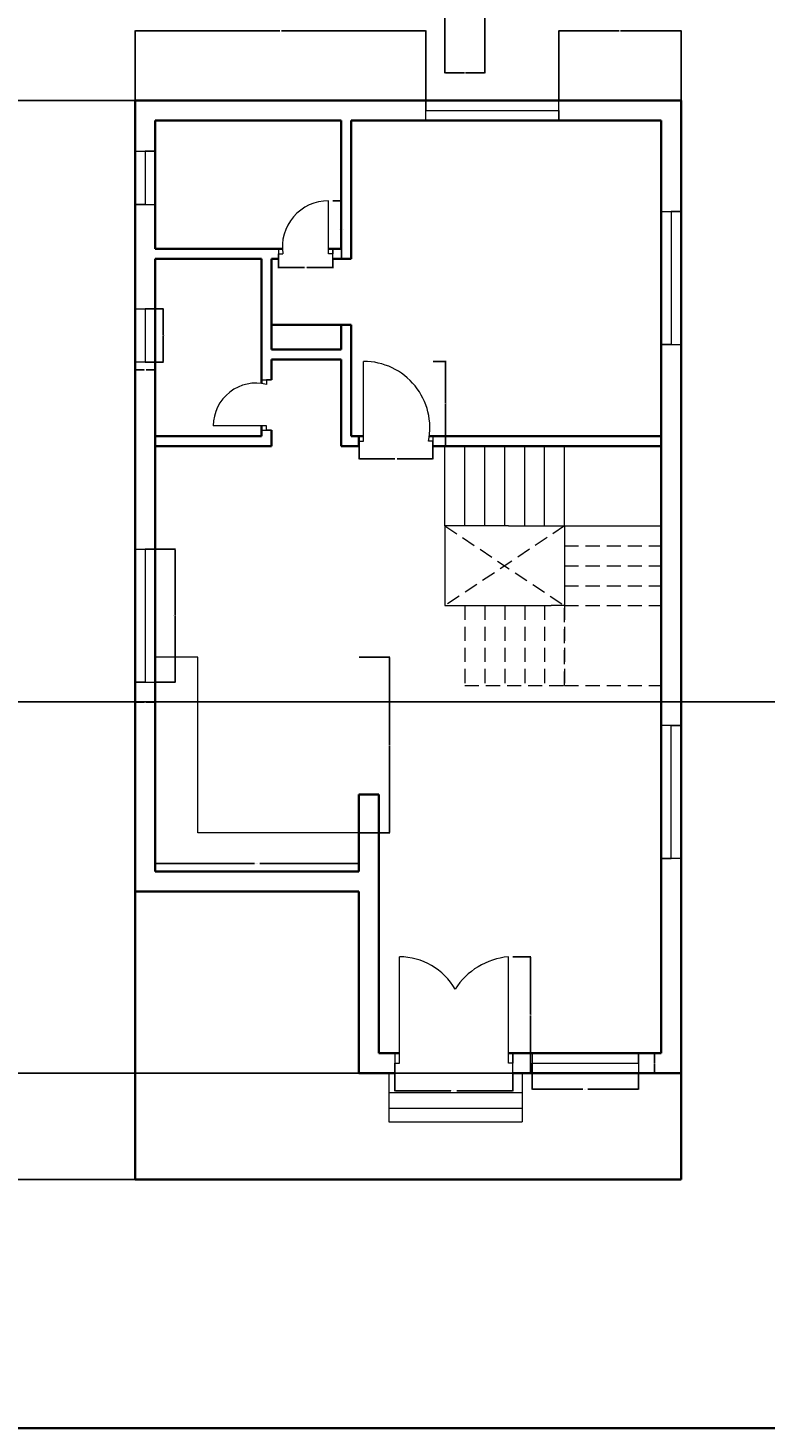
# Model space of a CAD drawing. Units: inches. Extents: x 1911 to 3278, y 2022 to 3108.
# Tile 11 of 13: x 2585 to 2918, y 2022 to 2654. Entities that reach past the tile are written whole.
import ezdxf

# ---------------------------------------------------------------- set-up
doc = ezdxf.new("R2010")
doc.units = ezdxf.units.IN
doc.linetypes.add('DASHED2', pattern=[9.525, 6.35, -3.175])
for name, color, linetype, lineweight in [('A-ANNO-DIMS', 2, 'Continuous', 18), ('A-ANNO-SYMB', 7, 'Continuous', 25), ('A-ANNO-TTLB', 7, 'Continuous', 35), ('A-DOOR', 4, 'Continuous', 18), ('A-FLOR-CASE', 9, 'Continuous', 18), ('A-FLOR-STRS', 7, 'Continuous', 18), ('A-FLOR-STRS-OVHD', 253, 'DASHED2', 13), ('A-GLAZ', 4, 'Continuous', 18), ('A-WALL', 7, 'Continuous', 35)]:
    doc.layers.add(name, color=color, linetype=linetype, lineweight=lineweight)
doc.styles.get("Standard").update_dxf_attribs({"font": 'arial.ttf'})
doc.dimstyles.get("Standard").update_dxf_attribs({"dimtxt": 0.18, "dimasz": 0.18, "dimexe": 0.18, "dimexo": 0.0625, "dimgap": 0.09, "dimtad": 0, "dimtih": 1, "dimtoh": 1, "dimdec": 4, "dimzin": 0, "dimdsep": 46, "dimtxsty": 'Standard', "dimcen": 0.09, "dimadec": 0, "dimazin": 0, "dimtfac": 1, "dimtdec": 4, "dimtofl": 0, "dimtmove": 0, "dimatfit": 3, "dimfxl": 1, "dimtolj": 1, "dimtzin": 0, "dimarcsym": 0})

# ---------------------------------------------------------------- blocks, each defined once
blk = doc.blocks.new('WIN-60')
for p, q in [((0, 60), (9, 60)), ((9, 60), (4.5, 60)), ((4.5, 60), (4.5, 0)), ((4.5, 0), (0, 0)), ((0, 0), (9, 0))]:
    blk.add_line(p, q)
blk = doc.blocks.new('WIN-24')
for p, q in [((0, 24), (9, 24)), ((9, 24), (4.5, 24)), ((4.5, 24), (4.5, 0)), ((4.5, 0), (0, 0)), ((0, 0), (9, 0))]:
    blk.add_line(p, q)
blk = doc.blocks.new('WIN-24-ALT-JAMB')
for p, q in [((0, 24), (9, 24)), ((9, 24), (4.5, 24)), ((4.5, 24), (4.5, 0)), ((9, 0), (0, 0)), ((4.5, 0), (9, 0))]:
    blk.add_line(p, q)
blk = doc.blocks.new('WIN-48')
for p, q in [((0, 9), (0, 0)), ((48, 4.5), (48, 9)), ((48, 9), (48, 0)), ((0, 0), (0, 4.5)), ((0, 4.5), (36, 4.5)), ((36, 4.5), (48, 4.5))]:
    blk.add_line(p, q)
blk = doc.blocks.new('DOOR-BATH-GF')
for p, q in [((22.54, 2.25), (22.54, 26.25)), ((0, 4.5), (0, 0)), ((0, 0), (0, 2.25)), ((0, 2.25), (2, 2.25)), ((24.54, 2.25), (22.54, 2.25)), ((24.54, 0), (24.54, 4.5)), ((24.54, 4.5), (24.54, 2.25))]:
    blk.add_line(p, q)
blk.add_arc((22.54, 5.46), 20.79, 90, 188.87385)
blk = doc.blocks.new('DOOR-WC-GF')
for p, q in [((21.75, 22.69), (26.25, 22.69)), ((26.25, 22.69), (24, 22.69)), ((24, 22.69), (24, 20.69)), ((24, 2), (0, 2)), ((24, 0), (24, 2)), ((21.75, 0), (26.25, 0)), ((26.25, 0), (24, 0))]:
    blk.add_line(p, q)
blk.add_arc((19.28, 2), 19.28, 75.82669, 180)
blk = doc.blocks.new('DOOR-BED-GF')
for p, q in [((2, 2.25), (2, 38.25)), ((0, 4.5), (0, 0)), ((0, 0), (0, 2.25)), ((0, 2.25), (0, 2.25)), ((0, 2.25), (2, 2.25)), ((33.28, 2.25), (31.28, 2.25)), ((33.28, 4.5), (33.28, 0)), ((33.28, 0), (33.28, 2.25))]:
    blk.add_line(p, q)
blk.add_arc((2, 8.34), 29.91, 348.25045, 90)
blk = doc.blocks.new('DOOR-ENTRY-PAIR')
for p, q in [((2, 40.5), (2, 52.5)), ((51.21, 4.5), (51.21, 52.5)), ((2, 4.5), (2, 40.5)), ((0, 9), (0, 0)), ((53.21, 0), (53.21, 9)), ((53.21, 9), (53.21, 4.5)), ((0, 0), (0, 4.5)), ((0, 4.5), (2, 4.5)), ((53.21, 4.5), (51.21, 4.5))]:
    blk.add_line(p, q)
for centre, radius, start, end in [((2, 23.47), 29.03, 29.81913, 90), ((54.01, 20.81), 31.81, 95.05335, 147.49255)]:
    blk.add_arc(centre, radius, start, end)
blk = doc.blocks.new('STEPS-ENTRY')
for p, q in [((0, 21.91), (0, 0)), ((60.1, 21.91), (60.1, 0)), ((0, 13.22), (60.1, 13.22)), ((60.1, 13.22), (60.1, 6)), ((60.1, 6), (0, 6)), ((0, 6), (0, 0)), ((0, 0), (60.1, 0))]:
    blk.add_line(p, q)
blk = doc.blocks.new('COUNTER-KITCHEN-L')
for p, q in [((19.27, 79.32), (0, 79.32)), ((19.27, 0), (19.27, 79.32)), ((92, 0), (19.27, 0))]:
    blk.add_line(p, q)
blk = doc.blocks.new('STAIR-PLAN-GF')
for p, q in [((0, 36), (0, 72)), ((9, 36), (9, 72)), ((18, 36), (18, 72)), ((27, 36), (27, 72)), ((36, 36), (36, 72)), ((45, 36), (45, 72)), ((54, 36), (54, 72)), ((28.63, 36), (0, 36)), ((0, 36), (0, 0)), ((28.63, 36), (97.65, 36)), ((54, 36), (54, 0)), ((54, 36), (54, 27)), ((0, 0), (48, 0)), ((54, 0), (48, 0))]:
    blk.add_line(p, q)
blk = doc.blocks.new('STAIR-BEYOND-GF')
for p, q in [((54, 72), (0, 36)), ((0, 72), (54, 36)), ((54, 72), (54, 63)), ((54, 63), (97.65, 63)), ((54, 54), (97.65, 54)), ((54, 45), (97.65, 45)), ((9, 36), (9, 0)), ((18, 36), (18, 0)), ((27, 36), (27, 0)), ((36, 36), (36, 0)), ((45, 36), (45, 0)), ((54, 36), (97.65, 36)), ((54, 0), (54, 36)), ((54, 36), (54, 0)), ((9, 0), (54, 0)), ((54, 0), (97.65, 0))]:
    blk.add_line(p, q)
blk = doc.blocks.new('*D24')
at = {"layer": 'A-ANNO-DIMS', "color": 0, "lineweight": -2, "transparency": 16777216}
for p, q in [((2642.42, 2418.3), (2651.53, 2418.3)), ((2651.35, 2418.12), (2651.35, 2388.48)), ((2651.35, 2358.48), (2651.35, 2388.12)), ((2642.42, 2358.3), (2651.53, 2358.3))]:
    blk.add_line(p, q, dxfattribs=at)
at = {"layer": 'A-ANNO-DIMS', "color": 0, "transparency": 16777216}
for points in [[(2651.32, 2418.12), (2651.38, 2418.12), (2651.35, 2418.3)], [(2651.32, 2358.48), (2651.38, 2358.48), (2651.35, 2358.3)]]:
    blk.add_solid(points, dxfattribs=at)
at = {"layer": 'Defpoints', "color": 0, "transparency": 16777216}
for p in [(2642.35, 2418.3), (2651.35, 2418.3), (2642.35, 2358.3)]:
    blk.add_point(p, dxfattribs=at)
at = {"layer": 'A-ANNO-DIMS', "color": 0, "transparency": 16777216, "insert": (2651.35, 2388.3), "char_height": 0.18, "attachment_point": 5}
blk.add_mtext('\\A1;WINDOW 60 TYP.', dxfattribs=at)
blk = doc.blocks.new('*D25')
at = {"layer": 'A-ANNO-DIMS', "color": 0, "lineweight": -2, "transparency": 16777216}
for p, q in [((2633.35, 2358.24), (2633.35, 2349.12)), ((2642.35, 2358.24), (2642.35, 2349.12)), ((2633.53, 2349.3), (2637.4, 2349.3)), ((2642.17, 2349.3), (2638.31, 2349.3))]:
    blk.add_line(p, q, dxfattribs=at)
at = {"layer": 'A-ANNO-DIMS', "color": 0, "transparency": 16777216}
for points in [[(2633.53, 2349.33), (2633.53, 2349.27), (2633.35, 2349.3)], [(2642.17, 2349.33), (2642.17, 2349.27), (2642.35, 2349.3)]]:
    blk.add_solid(points, dxfattribs=at)
at = {"layer": 'Defpoints', "color": 0, "transparency": 16777216}
for p in [(2633.35, 2358.3), (2642.35, 2358.3), (2642.35, 2349.3)]:
    blk.add_point(p, dxfattribs=at)
at = {"layer": 'A-ANNO-DIMS', "color": 0, "transparency": 16777216, "insert": (2637.85, 2349.3), "char_height": 0.18, "attachment_point": 5}
blk.add_mtext('\\A1;9 TYP.', dxfattribs=at)
blk = doc.blocks.new('*D28')
at = {"layer": 'A-ANNO-DIMS', "color": 0, "lineweight": -2, "transparency": 16777216}
for p, q in [((2642.42, 2526.84), (2646.13, 2526.84)), ((2645.95, 2526.66), (2645.95, 2515.02)), ((2645.95, 2503.02), (2645.95, 2514.66)), ((2642.42, 2502.84), (2646.13, 2502.84))]:
    blk.add_line(p, q, dxfattribs=at)
at = {"layer": 'A-ANNO-DIMS', "color": 0, "transparency": 16777216}
for points in [[(2645.92, 2526.66), (2645.98, 2526.66), (2645.95, 2526.84)], [(2645.92, 2503.02), (2645.98, 2503.02), (2645.95, 2502.84)]]:
    blk.add_solid(points, dxfattribs=at)
at = {"layer": 'Defpoints', "color": 0, "transparency": 16777216}
for p in [(2642.35, 2526.84), (2645.95, 2526.84), (2642.35, 2502.84)]:
    blk.add_point(p, dxfattribs=at)
at = {"layer": 'A-ANNO-DIMS', "color": 0, "transparency": 16777216, "insert": (2645.95, 2514.84), "char_height": 0.18, "attachment_point": 5}
blk.add_mtext('\\A1;ALT. JAMB 24 TYP.', dxfattribs=at)
blk = doc.blocks.new('*D29')
at = {"layer": 'A-ANNO-DIMS', "color": 0, "lineweight": -2, "transparency": 16777216}
for p, q in [((2633.35, 2502.78), (2633.35, 2499.06)), ((2642.35, 2502.78), (2642.35, 2499.06)), ((2633.53, 2499.24), (2637.4, 2499.24)), ((2642.17, 2499.24), (2638.31, 2499.24))]:
    blk.add_line(p, q, dxfattribs=at)
at = {"layer": 'A-ANNO-DIMS', "color": 0, "transparency": 16777216}
for points in [[(2633.53, 2499.27), (2633.53, 2499.21), (2633.35, 2499.24)], [(2642.17, 2499.27), (2642.17, 2499.21), (2642.35, 2499.24)]]:
    blk.add_solid(points, dxfattribs=at)
at = {"layer": 'Defpoints', "color": 0, "transparency": 16777216}
for p in [(2633.35, 2502.84), (2642.35, 2502.84), (2642.35, 2499.24)]:
    blk.add_point(p, dxfattribs=at)
at = {"layer": 'A-ANNO-DIMS', "color": 0, "transparency": 16777216, "insert": (2637.85, 2499.24), "char_height": 0.18, "attachment_point": 5}
blk.add_mtext('\\A1;9 TYP.', dxfattribs=at)
blk = doc.blocks.new('*D30')
at = {"layer": 'A-ANNO-DIMS', "color": 0, "lineweight": -2, "transparency": 16777216}
for p, q in [((2812.56, 2181.81), (2812.56, 2174.49)), ((2860.56, 2181.81), (2860.56, 2174.49)), ((2812.74, 2174.67), (2835.44, 2174.67)), ((2860.38, 2174.67), (2837.68, 2174.67))]:
    blk.add_line(p, q, dxfattribs=at)
at = {"layer": 'A-ANNO-DIMS', "color": 0, "transparency": 16777216}
for points in [[(2812.74, 2174.7), (2812.74, 2174.64), (2812.56, 2174.67)], [(2860.38, 2174.7), (2860.38, 2174.64), (2860.56, 2174.67)]]:
    blk.add_solid(points, dxfattribs=at)
at = {"layer": 'Defpoints', "color": 0, "transparency": 16777216}
for p in [(2812.56, 2181.87), (2860.56, 2181.87), (2860.56, 2174.67)]:
    blk.add_point(p, dxfattribs=at)
at = {"layer": 'A-ANNO-DIMS', "color": 0, "transparency": 16777216, "insert": (2836.56, 2174.67), "char_height": 0.18, "attachment_point": 5}
blk.add_mtext('\\A1;WINDOW 48 TYP.', dxfattribs=at)
blk = doc.blocks.new('*D31')
at = {"layer": 'A-ANNO-DIMS', "color": 0, "lineweight": -2, "transparency": 16777216}
for p, q in [((2860.62, 2190.87), (2867.94, 2190.87)), ((2867.76, 2190.69), (2867.76, 2186.56)), ((2860.62, 2181.87), (2867.94, 2181.87)), ((2867.76, 2182.05), (2867.76, 2186.19))]:
    blk.add_line(p, q, dxfattribs=at)
at = {"layer": 'A-ANNO-DIMS', "color": 0, "transparency": 16777216}
for points in [[(2867.73, 2190.69), (2867.79, 2190.69), (2867.76, 2190.87)], [(2867.73, 2182.05), (2867.79, 2182.05), (2867.76, 2181.87)]]:
    blk.add_solid(points, dxfattribs=at)
at = {"layer": 'Defpoints', "color": 0, "transparency": 16777216}
for p in [(2860.56, 2190.87), (2867.76, 2190.87), (2860.56, 2181.87)]:
    blk.add_point(p, dxfattribs=at)
at = {"layer": 'A-ANNO-DIMS', "color": 0, "transparency": 16777216, "insert": (2867.76, 2186.37), "char_height": 0.18, "attachment_point": 5}
blk.add_mtext('\\A1;9 TYP.', dxfattribs=at)
blk = doc.blocks.new('*D38')
at = {"layer": 'A-ANNO-DIMS', "color": 0, "lineweight": -2, "transparency": 16777216}
for p, q in [((2722.63, 2575.62), (2726.69, 2575.62)), ((2726.51, 2575.44), (2726.51, 2562.68)), ((2726.51, 2549.55), (2726.51, 2562.32)), ((2722.63, 2549.37), (2726.69, 2549.37))]:
    blk.add_line(p, q, dxfattribs=at)
at = {"layer": 'A-ANNO-DIMS', "color": 0, "transparency": 16777216}
for points in [[(2726.48, 2575.44), (2726.54, 2575.44), (2726.51, 2575.62)], [(2726.48, 2549.55), (2726.54, 2549.55), (2726.51, 2549.37)]]:
    blk.add_solid(points, dxfattribs=at)
at = {"layer": 'Defpoints', "color": 0, "transparency": 16777216}
for p in [(2722.57, 2575.62), (2726.51, 2575.62), (2722.57, 2549.37)]:
    blk.add_point(p, dxfattribs=at)
at = {"layer": 'A-ANNO-DIMS', "color": 0, "transparency": 16777216, "insert": (2726.51, 2562.5), "char_height": 0.18, "attachment_point": 5}
blk.add_mtext('\\A1;BATH DOOR 26 TYP.', dxfattribs=at)
blk = doc.blocks.new('*D39')
at = {"layer": 'A-ANNO-DIMS', "color": 0, "lineweight": -2, "transparency": 16777216}
for p, q in [((2698.03, 2549.31), (2698.03, 2545.26)), ((2722.57, 2549.31), (2722.57, 2545.26)), ((2698.21, 2545.44), (2709.77, 2545.44)), ((2722.39, 2545.44), (2710.83, 2545.44))]:
    blk.add_line(p, q, dxfattribs=at)
at = {"layer": 'A-ANNO-DIMS', "color": 0, "transparency": 16777216}
for points in [[(2698.21, 2545.47), (2698.21, 2545.41), (2698.03, 2545.44)], [(2722.39, 2545.47), (2722.39, 2545.41), (2722.57, 2545.44)]]:
    blk.add_solid(points, dxfattribs=at)
at = {"layer": 'Defpoints', "color": 0, "transparency": 16777216}
for p in [(2698.03, 2549.37), (2722.57, 2549.37), (2722.57, 2545.44)]:
    blk.add_point(p, dxfattribs=at)
at = {"layer": 'A-ANNO-DIMS', "color": 0, "transparency": 16777216, "insert": (2710.3, 2545.44), "char_height": 0.18, "attachment_point": 5}
blk.add_mtext('\\A1;25 TYP.', dxfattribs=at)
blk = doc.blocks.new('*D42')
at = {"layer": 'A-ANNO-DIMS', "color": 0, "lineweight": -2, "transparency": 16777216}
for p, q in [((2767.82, 2503.12), (2773.67, 2503.12)), ((2773.49, 2502.94), (2773.49, 2484.18)), ((2773.49, 2465.05), (2773.49, 2483.82)), ((2767.82, 2464.87), (2773.67, 2464.87))]:
    blk.add_line(p, q, dxfattribs=at)
at = {"layer": 'A-ANNO-DIMS', "color": 0, "transparency": 16777216}
for points in [[(2773.46, 2502.94), (2773.52, 2502.94), (2773.49, 2503.12)], [(2773.46, 2465.05), (2773.52, 2465.05), (2773.49, 2464.87)]]:
    blk.add_solid(points, dxfattribs=at)
at = {"layer": 'Defpoints', "color": 0, "transparency": 16777216}
for p in [(2767.76, 2503.12), (2773.49, 2503.12), (2767.76, 2464.87)]:
    blk.add_point(p, dxfattribs=at)
at = {"layer": 'A-ANNO-DIMS', "color": 0, "transparency": 16777216, "insert": (2773.49, 2484), "char_height": 0.18, "attachment_point": 5}
blk.add_mtext('\\A1;BEDROOM DOOR 38 TYP.', dxfattribs=at)
blk = doc.blocks.new('*D43')
at = {"layer": 'A-ANNO-DIMS', "color": 0, "lineweight": -2, "transparency": 16777216}
for p, q in [((2734.47, 2464.81), (2734.47, 2458.96)), ((2767.76, 2464.81), (2767.76, 2458.96)), ((2734.65, 2459.14), (2750.59, 2459.14)), ((2767.58, 2459.14), (2751.64, 2459.14))]:
    blk.add_line(p, q, dxfattribs=at)
at = {"layer": 'A-ANNO-DIMS', "color": 0, "transparency": 16777216}
for points in [[(2734.65, 2459.17), (2734.65, 2459.11), (2734.47, 2459.14)], [(2767.58, 2459.17), (2767.58, 2459.11), (2767.76, 2459.14)]]:
    blk.add_solid(points, dxfattribs=at)
at = {"layer": 'Defpoints', "color": 0, "transparency": 16777216}
for p in [(2734.47, 2464.87), (2767.76, 2464.87), (2767.76, 2459.14)]:
    blk.add_point(p, dxfattribs=at)
at = {"layer": 'A-ANNO-DIMS', "color": 0, "transparency": 16777216, "insert": (2751.12, 2459.14), "char_height": 0.18, "attachment_point": 5}
blk.add_mtext('\\A1;33 TYP.', dxfattribs=at)
blk = doc.blocks.new('*D44')
at = {"layer": 'A-ANNO-DIMS', "color": 0, "lineweight": -2, "transparency": 16777216}
for p, q in [((2750.62, 2181.81), (2750.62, 2173.71)), ((2803.83, 2181.81), (2803.83, 2173.71)), ((2750.8, 2173.89), (2775.92, 2173.89)), ((2803.65, 2173.89), (2778.54, 2173.89))]:
    blk.add_line(p, q, dxfattribs=at)
at = {"layer": 'A-ANNO-DIMS', "color": 0, "transparency": 16777216}
for points in [[(2750.8, 2173.92), (2750.8, 2173.86), (2750.62, 2173.89)], [(2803.65, 2173.92), (2803.65, 2173.86), (2803.83, 2173.89)]]:
    blk.add_solid(points, dxfattribs=at)
at = {"layer": 'Defpoints', "color": 0, "transparency": 16777216}
for p in [(2750.62, 2181.87), (2803.83, 2181.87), (2803.83, 2173.89)]:
    blk.add_point(p, dxfattribs=at)
at = {"layer": 'A-ANNO-DIMS', "color": 0, "transparency": 16777216, "insert": (2777.23, 2173.89), "char_height": 0.18, "attachment_point": 5}
blk.add_mtext('\\A1;ENTRY PAIR 53 TYP.', dxfattribs=at)
blk = doc.blocks.new('*D45')
at = {"layer": 'A-ANNO-DIMS', "color": 0, "lineweight": -2, "transparency": 16777216}
for p, q in [((2803.9, 2234.37), (2812, 2234.37)), ((2811.82, 2234.19), (2811.82, 2208.31)), ((2811.82, 2182.05), (2811.82, 2207.94)), ((2803.9, 2181.87), (2812, 2181.87))]:
    blk.add_line(p, q, dxfattribs=at)
at = {"layer": 'A-ANNO-DIMS', "color": 0, "transparency": 16777216}
for points in [[(2811.79, 2234.19), (2811.85, 2234.19), (2811.82, 2234.37)], [(2811.79, 2182.05), (2811.85, 2182.05), (2811.82, 2181.87)]]:
    blk.add_solid(points, dxfattribs=at)
at = {"layer": 'Defpoints', "color": 0, "transparency": 16777216}
for p in [(2803.83, 2234.37), (2811.82, 2234.37), (2803.83, 2181.87)]:
    blk.add_point(p, dxfattribs=at)
at = {"layer": 'A-ANNO-DIMS', "color": 0, "transparency": 16777216, "insert": (2811.82, 2208.12), "char_height": 0.18, "attachment_point": 5}
blk.add_mtext('\\A1;53 TYP.', dxfattribs=at)
blk = doc.blocks.new('*D58')
at = {"layer": 'A-ANNO-DIMS', "color": 0, "lineweight": -2, "transparency": 16777216}
for p, q in [((2642.35, 2290.21), (2642.35, 2276.29)), ((2734.35, 2290.21), (2734.35, 2276.29)), ((2642.53, 2276.47), (2687.17, 2276.47)), ((2734.17, 2276.47), (2689.54, 2276.47))]:
    blk.add_line(p, q, dxfattribs=at)
at = {"layer": 'A-ANNO-DIMS', "color": 0, "transparency": 16777216}
for points in [[(2642.53, 2276.5), (2642.53, 2276.44), (2642.35, 2276.47)], [(2734.17, 2276.5), (2734.17, 2276.44), (2734.35, 2276.47)]]:
    blk.add_solid(points, dxfattribs=at)
at = {"layer": 'Defpoints', "color": 0, "transparency": 16777216}
for p in [(2642.35, 2290.27), (2734.35, 2290.27), (2734.35, 2276.47)]:
    blk.add_point(p, dxfattribs=at)
at = {"layer": 'A-ANNO-DIMS', "color": 0, "transparency": 16777216, "insert": (2688.35, 2276.47), "char_height": 0.18, "attachment_point": 5}
blk.add_mtext('\\A1;COUNTER 92 TYP.', dxfattribs=at)
blk = doc.blocks.new('*D59')
at = {"layer": 'A-ANNO-DIMS', "color": 0, "lineweight": -2, "transparency": 16777216}
for p, q in [((2734.42, 2369.59), (2748.33, 2369.59)), ((2748.15, 2369.41), (2748.15, 2330.11)), ((2748.15, 2290.45), (2748.15, 2329.75)), ((2734.42, 2290.27), (2748.33, 2290.27))]:
    blk.add_line(p, q, dxfattribs=at)
at = {"layer": 'A-ANNO-DIMS', "color": 0, "transparency": 16777216}
for points in [[(2748.12, 2369.41), (2748.18, 2369.41), (2748.15, 2369.59)], [(2748.12, 2290.45), (2748.18, 2290.45), (2748.15, 2290.27)]]:
    blk.add_solid(points, dxfattribs=at)
at = {"layer": 'Defpoints', "color": 0, "transparency": 16777216}
for p in [(2734.35, 2369.59), (2748.15, 2369.59), (2734.35, 2290.27)]:
    blk.add_point(p, dxfattribs=at)
at = {"layer": 'A-ANNO-DIMS', "color": 0, "transparency": 16777216, "insert": (2748.15, 2329.93), "char_height": 0.18, "attachment_point": 5}
blk.add_mtext('\\A1;79 TYP.', dxfattribs=at)
blk = doc.blocks.new('*D81')
at = {"layer": 'A-ANNO-DIMS', "color": 0, "lineweight": -2, "transparency": 16777216}
for p, q in [((2633.35, 2620.94), (2633.35, 2652.45)), ((2633.53, 2652.27), (2698.57, 2652.27)), ((2764.37, 2652.27), (2699.34, 2652.27)), ((2764.55, 2620.94), (2764.55, 2652.45))]:
    blk.add_line(p, q, dxfattribs=at)
at = {"layer": 'A-ANNO-DIMS', "color": 0, "transparency": 16777216}
for points in [[(2633.53, 2652.3), (2633.53, 2652.24), (2633.35, 2652.27)], [(2764.37, 2652.3), (2764.37, 2652.24), (2764.55, 2652.27)]]:
    blk.add_solid(points, dxfattribs=at)
at = {"layer": 'Defpoints', "color": 0, "transparency": 16777216}
for p in [(2764.55, 2652.27), (2633.35, 2620.87), (2764.55, 2620.87)]:
    blk.add_point(p, dxfattribs=at)
at = {"layer": 'A-ANNO-DIMS', "color": 0, "transparency": 16777216, "insert": (2698.95, 2652.27), "char_height": 0.18, "attachment_point": 5}
blk.add_mtext('\\A1;131.2', dxfattribs=at)
blk = doc.blocks.new('*D82')
at = {"layer": 'A-ANNO-DIMS', "color": 0, "lineweight": -2, "transparency": 16777216}
for p, q in [((2824.55, 2620.94), (2824.55, 2652.45)), ((2824.73, 2652.27), (2851.88, 2652.27)), ((2879.67, 2652.27), (2852.53, 2652.27)), ((2879.85, 2620.94), (2879.85, 2652.45))]:
    blk.add_line(p, q, dxfattribs=at)
at = {"layer": 'A-ANNO-DIMS', "color": 0, "transparency": 16777216}
for points in [[(2824.73, 2652.3), (2824.73, 2652.24), (2824.55, 2652.27)], [(2879.67, 2652.3), (2879.67, 2652.24), (2879.85, 2652.27)]]:
    blk.add_solid(points, dxfattribs=at)
at = {"layer": 'Defpoints', "color": 0, "transparency": 16777216}
for p in [(2879.85, 2652.27), (2824.55, 2620.87), (2879.85, 2620.87)]:
    blk.add_point(p, dxfattribs=at)
at = {"layer": 'A-ANNO-DIMS', "color": 0, "transparency": 16777216, "insert": (2852.2, 2652.27), "char_height": 0.18, "attachment_point": 5}
blk.add_mtext('\\A1;55.3', dxfattribs=at)
blk = doc.blocks.new('*D83')
at = {"layer": 'A-ANNO-DIMS', "color": 0, "lineweight": -2, "transparency": 16777216}
for p, q in [((2633.29, 2620.87), (2561.76, 2620.87)), ((2561.94, 2620.69), (2561.94, 2485.38)), ((2561.94, 2349.71), (2561.94, 2485.02)), ((2593.28, 2349.53), (2561.76, 2349.53))]:
    blk.add_line(p, q, dxfattribs=at)
at = {"layer": 'A-ANNO-DIMS', "color": 0, "transparency": 16777216}
for points in [[(2561.91, 2620.69), (2561.97, 2620.69), (2561.94, 2620.87)], [(2561.91, 2349.71), (2561.97, 2349.71), (2561.94, 2349.53)]]:
    blk.add_solid(points, dxfattribs=at)
at = {"layer": 'Defpoints', "color": 0, "transparency": 16777216}
for p in [(2561.94, 2620.87), (2633.35, 2620.87), (2593.34, 2349.53)]:
    blk.add_point(p, dxfattribs=at)
at = {"layer": 'A-ANNO-DIMS', "color": 0, "transparency": 16777216, "insert": (2561.94, 2485.2), "char_height": 0.18, "attachment_point": 5}
blk.add_mtext('\\A1;271.35', dxfattribs=at)
blk = doc.blocks.new('*D87')
at = {"layer": 'A-ANNO-DIMS', "color": 0, "lineweight": -2, "transparency": 16777216}
for p, q in [((2593.28, 2349.53), (2561.76, 2349.53)), ((2561.94, 2349.35), (2561.94, 2241.88)), ((2561.94, 2134.05), (2561.94, 2241.52)), ((2633.29, 2133.87), (2561.76, 2133.87))]:
    blk.add_line(p, q, dxfattribs=at)
at = {"layer": 'A-ANNO-DIMS', "color": 0, "transparency": 16777216}
for points in [[(2561.91, 2349.35), (2561.97, 2349.35), (2561.94, 2349.53)], [(2561.91, 2134.05), (2561.97, 2134.05), (2561.94, 2133.87)]]:
    blk.add_solid(points, dxfattribs=at)
at = {"layer": 'Defpoints', "color": 0, "transparency": 16777216}
for p in [(2593.34, 2349.53), (2561.94, 2133.87), (2633.35, 2133.87)]:
    blk.add_point(p, dxfattribs=at)
at = {"layer": 'A-ANNO-DIMS', "color": 0, "transparency": 16777216, "insert": (2561.94, 2241.7), "char_height": 0.18, "attachment_point": 5}
blk.add_mtext('\\A1;215.65', dxfattribs=at)
blk = doc.blocks.new('*D88')
at = {"layer": 'A-ANNO-DIMS', "color": 0, "lineweight": -2, "transparency": 16777216}
for p, q in [((2879.79, 2181.87), (2561.76, 2181.87)), ((2561.94, 2181.69), (2561.94, 2158.06)), ((2561.94, 2134.05), (2561.94, 2157.69)), ((2879.79, 2133.87), (2561.76, 2133.87))]:
    blk.add_line(p, q, dxfattribs=at)
at = {"layer": 'A-ANNO-DIMS', "color": 0, "transparency": 16777216}
for points in [[(2561.91, 2181.69), (2561.97, 2181.69), (2561.94, 2181.87)], [(2561.91, 2134.05), (2561.97, 2134.05), (2561.94, 2133.87)]]:
    blk.add_solid(points, dxfattribs=at)
at = {"layer": 'Defpoints', "color": 0, "transparency": 16777216}
for p in [(2561.94, 2181.87), (2879.85, 2181.87), (2879.85, 2133.87)]:
    blk.add_point(p, dxfattribs=at)
at = {"layer": 'A-ANNO-DIMS', "color": 0, "transparency": 16777216, "insert": (2561.94, 2157.87), "char_height": 0.18, "attachment_point": 5}
blk.add_mtext('\\A1;48', dxfattribs=at)
blk = doc.blocks.new('*D99')
at = {"layer": 'A-ANNO-DIMS', "color": 0, "lineweight": -2, "transparency": 16777216}
for p, q in [((2773.2, 2733.96), (2773.2, 2633.15)), ((2791.2, 2733.96), (2791.2, 2633.15)), ((2773.38, 2633.33), (2781.99, 2633.33)), ((2791.02, 2633.33), (2782.42, 2633.33))]:
    blk.add_line(p, q, dxfattribs=at)
at = {"layer": 'A-ANNO-DIMS', "color": 0, "transparency": 16777216}
for points in [[(2773.38, 2633.36), (2773.38, 2633.3), (2773.2, 2633.33)], [(2791.02, 2633.36), (2791.02, 2633.3), (2791.2, 2633.33)]]:
    blk.add_solid(points, dxfattribs=at)
at = {"layer": 'Defpoints', "color": 0, "transparency": 16777216}
for p in [(2773.2, 2734.03), (2791.2, 2734.03), (2791.2, 2633.33)]:
    blk.add_point(p, dxfattribs=at)
at = {"layer": 'A-ANNO-DIMS', "color": 0, "transparency": 16777216, "insert": (2782.2, 2633.33), "char_height": 0.18, "attachment_point": 5}
blk.add_mtext('\\A1;18', dxfattribs=at)

msp = doc.modelspace()

# ---------------------------------------------------------------- linework, layer by layer
at = {"layer": 'A-ANNO-SYMB'}
msp.add_line((3195.5436, 2349.5267), (2593.3449, 2349.5267), dxfattribs=at)
at = {"layer": 'A-ANNO-TTLB'}
msp.add_lwpolyline([(1911.3875, 3108.0628), (3278.3142, 3108.0628), (3278.3142, 2021.7237), (1911.3875, 2021.7237)], close=True, dxfattribs=at)
at = {"layer": 'A-WALL'}
for p, q in [((2633.3539, 2620.8733), (2633.3539, 2133.8733)), ((2633.3539, 2620.8733), (2633.3539, 2133.8733)), ((2633.3539, 2620.8733), (2879.8539, 2620.8733)), ((2879.8539, 2620.8733), (2879.8539, 2133.8733)), ((2642.3539, 2611.8733), (2642.3539, 2553.8733)), ((2642.3539, 2611.8733), (2726.3539, 2611.8733)), ((2726.3539, 2611.8733), (2726.3539, 2553.8733)), ((2730.8539, 2611.8733), (2730.8539, 2549.3733)), ((2730.8539, 2611.8733), (2870.8539, 2611.8733)), ((2870.8539, 2611.8733), (2870.8539, 2226.8733)), ((2642.3539, 2553.8733), (2699.8, 2553.8733)), ((2720.5705, 2553.8733), (2726.3539, 2553.8733)), ((2642.3539, 2549.3733), (2642.3539, 2272.8733)), ((2642.3539, 2549.3733), (2690.3539, 2549.3733)), ((2690.3539, 2549.3733), (2690.3539, 2493.1601)), ((2694.8539, 2549.3733), (2694.8539, 2508.4462)), ((2694.8539, 2549.3733), (2698.0268, 2549.3733)), ((2722.5705, 2549.3733), (2730.8539, 2549.3733)), ((2726.3539, 2519.5634), (2694.8539, 2519.5634)), ((2730.8539, 2519.5634), (2726.3539, 2519.5634)), ((2726.3539, 2519.5634), (2726.3539, 2508.4462)), ((2730.8539, 2508.4462), (2730.8539, 2519.5634)), ((2726.3539, 2508.4462), (2694.8539, 2508.4462)), ((2694.8539, 2503.9462), (2694.8539, 2494.7321)), ((2694.8539, 2503.9462), (2726.3539, 2503.9462)), ((2726.3539, 2503.9462), (2726.3539, 2464.8733)), ((2730.8539, 2508.4462), (2730.8539, 2469.3733)), ((2690.3539, 2474.0397), (2690.3539, 2469.3733)), ((2694.8539, 2472.0397), (2694.8539, 2464.8733)), ((2642.3539, 2469.3733), (2690.3539, 2469.3733)), ((2642.3539, 2464.8733), (2694.8539, 2464.8733)), ((2730.8539, 2464.8733), (2726.3539, 2464.8733)), ((2730.8539, 2469.3733), (2736.4743, 2469.3733)), ((2730.8539, 2464.8733), (2734.4743, 2464.8733)), ((2734.3539, 2469.3733), (2734.3539, 2464.8733)), ((2766.1361, 2469.3733), (2870.8539, 2469.3733)), ((2767.757, 2464.8733), (2870.8539, 2464.8733)), ((2743.3539, 2307.6624), (2734.3539, 2307.6624)), ((2734.3539, 2307.6624), (2734.3539, 2272.8733)), ((2743.3539, 2272.8733), (2743.3539, 2307.6624)), ((2642.3539, 2272.8733), (2734.3539, 2272.8733)), ((2743.3539, 2272.8733), (2743.3539, 2226.8733)), ((2633.3539, 2263.8733), (2734.3539, 2263.8733)), ((2734.3539, 2263.8733), (2734.3539, 2217.8733)), ((2743.3539, 2190.8733), (2743.3539, 2226.8733)), ((2870.8539, 2226.8733), (2870.8539, 2190.8733)), ((2734.3539, 2217.8733), (2734.3539, 2181.8733)), ((2752.6229, 2190.8733), (2743.3539, 2190.8733)), ((2801.8341, 2190.8733), (2870.8539, 2190.8733)), ((2734.3539, 2181.8733), (2750.6229, 2181.8733)), ((2803.8341, 2181.8733), (2879.8539, 2181.8733)), ((2633.3539, 2133.8733), (2743.3539, 2133.8733)), ((2743.3539, 2133.8733), (2879.8539, 2133.8733))]:
    msp.add_line(p, q, dxfattribs=at)

# ---------------------------------------------------------------- block references
at = {"layer": 'A-DOOR'}
for name, p in [('DOOR-BATH-GF', (2698.0265, 2549.373)), ('DOOR-BED-GF', (2734.4745, 2464.873)), ('DOOR-WC-GF', (2668.6035, 2472.04)), ('DOOR-ENTRY-PAIR', (2750.6225, 2181.873))]:
    msp.add_blockref(name, p, dxfattribs=at)
at = {"layer": 'A-FLOR-CASE'}
msp.add_blockref('COUNTER-KITCHEN-L', (2642.3535, 2290.268), dxfattribs=at)
at = {"layer": 'A-FLOR-STRS'}
for name, p in [('STAIR-PLAN-GF', (2773.2045, 2392.873)), ('STEPS-ENTRY', (2747.9075, 2159.968))]:
    msp.add_blockref(name, p, dxfattribs=at)
at = {"layer": 'A-FLOR-STRS-OVHD'}
msp.add_blockref('STAIR-BEYOND-GF', (2773.2045, 2356.873), dxfattribs=at)
at = {"layer": 'A-GLAZ'}
for p, rotation in [((2824.5526, 2611.8729), 90.00000000000286), ((2879.8543, 2338.712), 180)]:
    msp.add_blockref('WIN-60', p, dxfattribs=dict(at, rotation=rotation))
for name, p in [('WIN-24', (2633.3535, 2573.942)), ('WIN-60', (2870.8535, 2510.7737)), ('WIN-24-ALT-JAMB', (2633.3535, 2502.841)), ('WIN-60', (2633.3535, 2358.3)), ('WIN-48', (2812.5605, 2181.873))]:
    msp.add_blockref(name, p, dxfattribs=at)

# ---------------------------------------------------------------- dimensions: what is measured, and where the dimension line sits
at = {"layer": 'A-ANNO-DIMS'}
for base, p1, p2, override, picture, middle in [((2791.2046, 2633.3258), (2773.2046, 2734.0271), (2791.2046, 2734.0271), {"dimdec": 0, "dimlfac": 1, "dimrnd": 0, "dimzin": 0, "dimdsep": 46, "dimlunit": 2}, '*D99', (2782.2046, 2633.3258)), ((2764.5523, 2652.2733), (2633.3539, 2620.8733), (2764.5523, 2620.8733), {"dimdec": 1, "dimlfac": 1, "dimrnd": 0, "dimzin": 0, "dimdsep": 46, "dimlunit": 2}, '*D81', (2698.9531, 2652.2733)), ((2879.8539, 2652.2733), (2824.5523, 2620.8733), (2879.8539, 2620.8733), {"dimdec": 1, "dimlfac": 1, "dimrnd": 0, "dimzin": 0, "dimdsep": 46, "dimlunit": 2}, '*D82', (2852.2031, 2652.2733))]:
    dim = msp.add_linear_dim(base=base, p1=p1, p2=p2, dimstyle='Standard', override=override, dxfattribs=at)
    dim.commit()
    dim.dimension.update_dxf_attribs({"geometry": picture, "text_midpoint": middle})
for base, p1, p2, override, picture, middle in [((2561.9449, 2620.8733), (2593.3449, 2349.5267), (2633.3539, 2620.8733), {"dimdec": 2, "dimlfac": 1, "dimrnd": 0, "dimzin": 0, "dimdsep": 46, "dimlunit": 2}, '*D83', (2561.9449, 2485.2)), ((2561.9449, 2133.8733), (2593.3449, 2349.5267), (2633.3539, 2133.8733), {"dimdec": 2, "dimlfac": 1, "dimrnd": 0, "dimzin": 0, "dimdsep": 46, "dimlunit": 2}, '*D87', (2561.9449, 2241.7)), ((2561.9449, 2181.8733), (2879.8539, 2133.8733), (2879.8539, 2181.8733), {"dimdec": 0, "dimlfac": 1, "dimrnd": 0, "dimzin": 0, "dimdsep": 46, "dimlunit": 2}, '*D88', (2561.9449, 2157.8733))]:
    dim = msp.add_linear_dim(base=base, p1=p1, p2=p2, angle=90, dimstyle='Standard', override=override, dxfattribs=at)
    dim.commit()
    dim.dimension.update_dxf_attribs({"geometry": picture, "text_midpoint": middle})
for base, p1, p2, text, picture, middle in [((2726.508, 2575.6233), (2722.5705, 2549.3733), (2722.5705, 2575.6233), 'BATH DOOR <> TYP.', '*D38', (2726.508, 2562.4983)), ((2645.9539, 2526.8406), (2642.3539, 2502.8406), (2642.3539, 2526.8406), 'ALT. JAMB <> TYP.', '*D28', (2645.9539, 2514.8406)), ((2773.4945, 2503.1233), (2767.757, 2464.8733), (2767.757, 2503.1233), 'BEDROOM DOOR <> TYP.', '*D42', (2773.4945, 2483.9983)), ((2651.3539, 2418.3003), (2642.3539, 2358.3003), (2642.3539, 2418.3003), 'WINDOW <> TYP.', '*D24', (2651.3539, 2388.3003)), ((2748.1539, 2369.589), (2734.3539, 2290.2678), (2734.3539, 2369.589), '<> TYP.', '*D59', (2748.1539, 2329.9284)), ((2811.8157954051, 2234.3732928528), (2803.8341165474, 2181.8732928528), (2803.8341165474, 2234.3732928528), '<> TYP.', '*D45', (2811.8157954051, 2208.1232928528)), ((2867.7601, 2190.8733), (2860.5601, 2181.8733), (2860.5601, 2190.8733), '<> TYP.', '*D31', (2867.7601, 2186.3733))]:
    dim = msp.add_linear_dim(base=base, p1=p1, p2=p2, angle=90, text=text, dimstyle='Standard', override={"dimdec": 0, "dimlfac": 1, "dimrnd": 0, "dimzin": 0, "dimdsep": 46, "dimlunit": 2}, dxfattribs=at)
    dim.commit()
    dim.dimension.update_dxf_attribs({"geometry": picture, "text_midpoint": middle})
for base, p1, p2, text, picture, middle in [((2722.5705, 2545.4358), (2698.0268, 2549.3733), (2722.5705, 2549.3733), '<> TYP.', '*D39', (2710.2986, 2545.4358)), ((2642.3539, 2499.2406), (2633.3539, 2502.8406), (2642.3539, 2502.8406), '<> TYP.', '*D29', (2637.8539, 2499.2406)), ((2767.757, 2459.1358), (2734.4743, 2464.8733), (2767.757, 2464.8733), '<> TYP.', '*D43', (2751.1156, 2459.1358)), ((2642.3539, 2349.3003), (2633.3539, 2358.3003), (2642.3539, 2358.3003), '<> TYP.', '*D25', (2637.8539, 2349.3003)), ((2734.3539, 2276.4678), (2642.3539, 2290.2678), (2734.3539, 2290.2678), 'COUNTER <> TYP.', '*D58', (2688.3539, 2276.4678)), ((2803.8341, 2173.8916), (2750.6229, 2181.8733), (2803.8341, 2181.8733), 'ENTRY PAIR <> TYP.', '*D44', (2777.2285, 2173.8916)), ((2860.5601, 2174.6733), (2812.5601, 2181.8733), (2860.5601, 2181.8733), 'WINDOW <> TYP.', '*D30', (2836.5601, 2174.6733))]:
    dim = msp.add_linear_dim(base=base, p1=p1, p2=p2, text=text, dimstyle='Standard', override={"dimdec": 0, "dimlfac": 1, "dimrnd": 0, "dimzin": 0, "dimdsep": 46, "dimlunit": 2}, dxfattribs=at)
    dim.commit()
    dim.dimension.update_dxf_attribs({"geometry": picture, "text_midpoint": middle})

doc.saveas('drawing.dxf')
